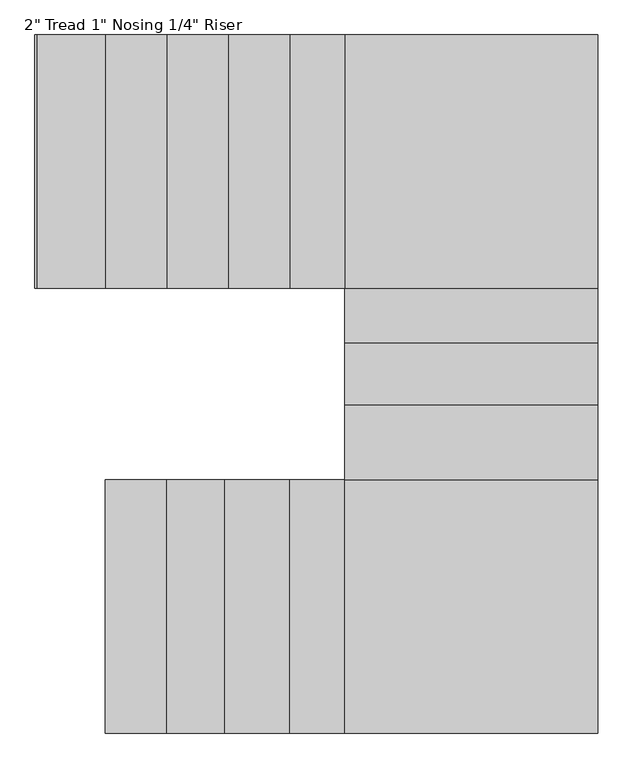
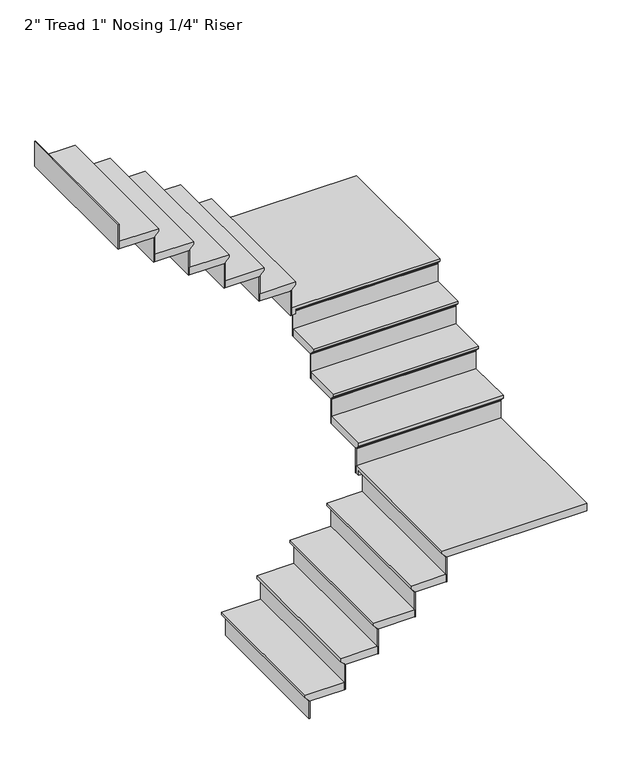
"""IFC4 building model written with IfcOpenShell, lengths in millimetres: stair flight geometry."""

from ifc_helpers import new_model, si_unit, origin, place, context, project, spatial, faceted_brep, source, transform, mapped, element, save


def stair_flight_f19c2654(model_context):
    return source(origin(), model_context, "Body", "Brep", [
        faceted_brep([(344.764115, -6141.1350571, 9751.4833333), (344.764115, -6141.1350571, 9770.5333333), (344.764115, -5201.3350571, 9770.5333333), (344.764115, -5201.3350571, 9751.4833333), (370.164115, -6141.1350571, 9726.0833333), (370.164115, -5201.3350571, 9726.0833333), (598.764115, -6141.1350571, 9770.5333333), (598.764115, -5201.3350571, 9770.5333333), (370.164115, -5201.3350571, 9719.7333333), (598.764115, -5201.3350571, 9719.7333333), (598.764115, -6141.1350571, 9719.7333333), (370.164115, -6141.1350571, 9719.7333333)], [[[0, 1, 2, 3]], [[4, 0, 3, 5]], [[2, 1, 6, 7]], [[8, 9, 10, 11]], [[2, 7, 9, 8, 5, 3]], [[8, 11, 4, 5]], [[6, 1, 0, 4, 11, 10]], [[7, 6, 10, 9]]]),
        faceted_brep([(370.164115, -6141.1350571, 9719.7333333), (370.164115, -6141.1350571, 9601.2), (376.514115, -6141.1350571, 9601.2), (376.514115, -6141.1350571, 9719.7333333), (370.164115, -5201.3350571, 9719.7333333), (376.514115, -5201.3350571, 9719.7333333), (376.514115, -5201.3350571, 9601.2), (370.164115, -5201.3350571, 9601.2)], [[[0, 1, 2, 3]], [[4, 5, 6, 7]], [[1, 0, 4, 7]], [[2, 1, 7, 6]], [[3, 2, 6, 5]], [[0, 3, 5, 4]]]),
        faceted_brep([(598.764115, -6141.1350571, 9889.0666667), (598.764115, -6141.1350571, 9719.7333333), (605.114115, -6141.1350571, 9719.7333333), (605.114115, -6141.1350571, 9889.0666667), (598.764115, -5201.3350571, 9889.0666667), (605.114115, -5201.3350571, 9889.0666667), (605.114115, -5201.3350571, 9719.7333333), (598.764115, -5201.3350571, 9719.7333333)], [[[0, 1, 2, 3]], [[4, 5, 6, 7]], [[1, 0, 4, 7]], [[2, 1, 7, 6]], [[3, 2, 6, 5]], [[0, 3, 5, 4]]]),
        faceted_brep([(573.364115, -5201.3350571, 9939.8666667), (573.364115, -6141.1350571, 9939.8666667), (814.664115, -6141.1350571, 9939.8666667), (814.664115, -5201.3350571, 9939.8666667), (598.764115, -5201.3350571, 9889.0666667), (814.664115, -5201.3350571, 9889.0666667), (814.664115, -6141.1350571, 9889.0666667), (598.764115, -6141.1350571, 9889.0666667), (598.764115, -5201.3350571, 9895.4166667), (573.364115, -5201.3350571, 9920.8166667), (598.764115, -6141.1350571, 9895.4166667), (573.364115, -6141.1350571, 9920.8166667)], [[[0, 1, 2, 3]], [[4, 5, 6, 7]], [[0, 3, 5, 4, 8, 9]], [[4, 7, 10, 8]], [[2, 1, 11, 10, 7, 6]], [[3, 2, 6, 5]], [[11, 1, 0, 9]], [[10, 11, 9, 8]]]),
        faceted_brep([(814.664115, -6141.1350571, 10058.4), (814.664115, -6141.1350571, 9889.0666667), (821.014115, -6141.1350571, 9889.0666667), (821.014115, -6141.1350571, 10058.4), (814.664115, -5201.3350571, 10058.4), (821.014115, -5201.3350571, 10058.4), (821.014115, -5201.3350571, 9889.0666667), (814.664115, -5201.3350571, 9889.0666667)], [[[0, 1, 2, 3]], [[4, 5, 6, 7]], [[1, 0, 4, 7]], [[2, 1, 7, 6]], [[3, 2, 6, 5]], [[0, 3, 5, 4]]]),
        faceted_brep([(789.264115, -5201.3350571, 10109.2), (789.264115, -6141.1350571, 10109.2), (1055.964115, -6141.1350571, 10109.2), (1055.964115, -5201.3350571, 10109.2), (814.664115, -5201.3350571, 10058.4), (1055.964115, -5201.3350571, 10058.4), (1055.964115, -6141.1350571, 10058.4), (814.664115, -6141.1350571, 10058.4), (814.664115, -5201.3350571, 10064.75), (789.264115, -5201.3350571, 10090.15), (814.664115, -6141.1350571, 10064.75), (789.264115, -6141.1350571, 10090.15)], [[[0, 1, 2, 3]], [[4, 5, 6, 7]], [[0, 3, 5, 4, 8, 9]], [[4, 7, 10, 8]], [[2, 1, 11, 10, 7, 6]], [[3, 2, 6, 5]], [[11, 1, 0, 9]], [[10, 11, 9, 8]]]),
        faceted_brep([(1055.964115, -6141.1350571, 10227.7333333), (1055.964115, -6141.1350571, 10058.4), (1062.314115, -6141.1350571, 10058.4), (1062.314115, -6141.1350571, 10227.7333333), (1055.964115, -5201.3350571, 10227.7333333), (1062.314115, -5201.3350571, 10227.7333333), (1062.314115, -5201.3350571, 10058.4), (1055.964115, -5201.3350571, 10058.4)], [[[0, 1, 2, 3]], [[4, 5, 6, 7]], [[1, 0, 4, 7]], [[2, 1, 7, 6]], [[3, 2, 6, 5]], [[0, 3, 5, 4]]]),
        faceted_brep([(1030.564115, -5201.3350571, 10278.5333333), (1030.564115, -6141.1350571, 10278.5333333), (1259.164115, -6141.1350571, 10278.5333333), (1259.164115, -5201.3350571, 10278.5333333), (1055.964115, -5201.3350571, 10227.7333333), (1259.164115, -5201.3350571, 10227.7333333), (1259.164115, -6141.1350571, 10227.7333333), (1055.964115, -6141.1350571, 10227.7333333), (1055.964115, -5201.3350571, 10234.0833333), (1030.564115, -5201.3350571, 10259.4833333), (1055.964115, -6141.1350571, 10234.0833333), (1030.564115, -6141.1350571, 10259.4833333)], [[[0, 1, 2, 3]], [[4, 5, 6, 7]], [[0, 3, 5, 4, 8, 9]], [[4, 7, 10, 8]], [[2, 1, 11, 10, 7, 6]], [[3, 2, 6, 5]], [[11, 1, 0, 9]], [[10, 11, 9, 8]]]),
        faceted_brep([(1259.164115, -6141.1350571, 10397.0666667), (1259.164115, -6141.1350571, 10227.7333333), (1265.514115, -6141.1350571, 10227.7333333), (1265.514115, -6141.1350571, 10397.0666667), (1259.164115, -5201.3350571, 10397.0666667), (1265.514115, -5201.3350571, 10397.0666667), (1265.514115, -5201.3350571, 10227.7333333), (1259.164115, -5201.3350571, 10227.7333333)], [[[0, 1, 2, 3]], [[4, 5, 6, 7]], [[1, 0, 4, 7]], [[2, 1, 7, 6]], [[3, 2, 6, 5]], [[0, 3, 5, 4]]]),
        faceted_brep([(2173.564115, -6141.1350571, 10447.8666667), (2173.564115, -5175.9350571, 10447.8666667), (1233.764115, -5175.9350571, 10447.8666667), (1233.764115, -6141.1350571, 10447.8666667), (1233.764115, -5201.3350571, 10397.0666667), (1233.764115, -5175.9350571, 10397.0666667), (2173.564115, -5175.9350571, 10397.0666667), (2173.564115, -6141.1350571, 10397.0666667), (1259.164115, -6141.1350571, 10397.0666667), (1259.164115, -5201.3350571, 10397.0666667), (1233.764115, -5201.3350571, 10428.8166667), (1233.764115, -6141.1350571, 10428.8166667), (1259.164115, -5201.3350571, 10403.4166667), (1259.164115, -6141.1350571, 10403.4166667)], [[[0, 1, 2, 3]], [[4, 5, 6, 7, 8, 9]], [[3, 2, 5, 4, 10, 11]], [[4, 9, 12, 10]], [[9, 8, 13, 12]], [[0, 3, 11, 13, 8, 7]], [[1, 0, 7, 6]], [[2, 1, 6, 5]], [[13, 11, 10, 12]]]),
        faceted_brep([(2173.564115, -5175.9350571, 10566.4), (2173.564115, -5175.9350571, 10397.0666667), (2173.564115, -5169.5850571, 10397.0666667), (2173.564115, -5169.5850571, 10566.4), (1233.764115, -5175.9350571, 10566.4), (1233.764115, -5169.5850571, 10566.4), (1233.764115, -5169.5850571, 10397.0666667), (1233.764115, -5175.9350571, 10397.0666667)], [[[0, 1, 2, 3]], [[4, 5, 6, 7]], [[1, 0, 4, 7]], [[2, 1, 7, 6]], [[3, 2, 6, 5]], [[0, 3, 5, 4]]]),
        faceted_brep([(1233.764115, -5201.3350571, 10617.2), (2173.564115, -5201.3350571, 10617.2), (2173.564115, -4896.5350571, 10617.2), (1233.764115, -4896.5350571, 10617.2), (1233.764115, -5175.9350571, 10566.4), (1233.764115, -4896.5350571, 10566.4), (2173.564115, -4896.5350571, 10566.4), (2173.564115, -5175.9350571, 10566.4), (1233.764115, -5175.9350571, 10572.75), (1233.764115, -5201.3350571, 10598.15), (2173.564115, -5175.9350571, 10572.75), (2173.564115, -5201.3350571, 10598.15)], [[[0, 1, 2, 3]], [[4, 5, 6, 7]], [[0, 3, 5, 4, 8, 9]], [[4, 7, 10, 8]], [[2, 1, 11, 10, 7, 6]], [[3, 2, 6, 5]], [[11, 1, 0, 9]], [[10, 11, 9, 8]]]),
        faceted_brep([(2173.564115, -4896.5350571, 10735.7333333), (2173.564115, -4896.5350571, 10566.4), (2173.564115, -4890.1850571, 10566.4), (2173.564115, -4890.1850571, 10735.7333333), (1233.764115, -4896.5350571, 10735.7333333), (1233.764115, -4890.1850571, 10735.7333333), (1233.764115, -4890.1850571, 10566.4), (1233.764115, -4896.5350571, 10566.4)], [[[0, 1, 2, 3]], [[4, 5, 6, 7]], [[1, 0, 4, 7]], [[2, 1, 7, 6]], [[3, 2, 6, 5]], [[0, 3, 5, 4]]]),
        faceted_brep([(1233.764115, -4921.9350571, 10786.5333333), (2173.564115, -4921.9350571, 10786.5333333), (2173.564115, -4667.9350571, 10786.5333333), (1233.764115, -4667.9350571, 10786.5333333), (1233.764115, -4896.5350571, 10735.7333333), (1233.764115, -4667.9350571, 10735.7333333), (2173.564115, -4667.9350571, 10735.7333333), (2173.564115, -4896.5350571, 10735.7333333), (1233.764115, -4896.5350571, 10742.0833333), (1233.764115, -4921.9350571, 10767.4833333), (2173.564115, -4896.5350571, 10742.0833333), (2173.564115, -4921.9350571, 10767.4833333)], [[[0, 1, 2, 3]], [[4, 5, 6, 7]], [[0, 3, 5, 4, 8, 9]], [[4, 7, 10, 8]], [[2, 1, 11, 10, 7, 6]], [[3, 2, 6, 5]], [[11, 1, 0, 9]], [[10, 11, 9, 8]]]),
        faceted_brep([(2173.564115, -4667.9350571, 10905.0666667), (2173.564115, -4667.9350571, 10735.7333333), (2173.564115, -4661.5850571, 10735.7333333), (2173.564115, -4661.5850571, 10905.0666667), (1233.764115, -4667.9350571, 10905.0666667), (1233.764115, -4661.5850571, 10905.0666667), (1233.764115, -4661.5850571, 10735.7333333), (1233.764115, -4667.9350571, 10735.7333333)], [[[0, 1, 2, 3]], [[4, 5, 6, 7]], [[1, 0, 4, 7]], [[2, 1, 7, 6]], [[3, 2, 6, 5]], [[0, 3, 5, 4]]]),
        faceted_brep([(1233.764115, -4693.3350571, 10955.8666667), (2173.564115, -4693.3350571, 10955.8666667), (2173.564115, -4464.7350571, 10955.8666667), (1233.764115, -4464.7350571, 10955.8666667), (1233.764115, -4667.9350571, 10905.0666667), (1233.764115, -4464.7350571, 10905.0666667), (2173.564115, -4464.7350571, 10905.0666667), (2173.564115, -4667.9350571, 10905.0666667), (1233.764115, -4667.9350571, 10911.4166667), (1233.764115, -4693.3350571, 10936.8166667), (2173.564115, -4667.9350571, 10911.4166667), (2173.564115, -4693.3350571, 10936.8166667)], [[[0, 1, 2, 3]], [[4, 5, 6, 7]], [[0, 3, 5, 4, 8, 9]], [[4, 7, 10, 8]], [[2, 1, 11, 10, 7, 6]], [[3, 2, 6, 5]], [[11, 1, 0, 9]], [[10, 11, 9, 8]]]),
        faceted_brep([(2173.564115, -4464.7350571, 11074.4), (2173.564115, -4464.7350571, 10905.0666667), (2173.564115, -4458.3850571, 10905.0666667), (2173.564115, -4458.3850571, 11074.4), (1233.764115, -4464.7350571, 11074.4), (1233.764115, -4458.3850571, 11074.4), (1233.764115, -4458.3850571, 10905.0666667), (1233.764115, -4464.7350571, 10905.0666667)], [[[0, 1, 2, 3]], [[4, 5, 6, 7]], [[1, 0, 4, 7]], [[2, 1, 7, 6]], [[3, 2, 6, 5]], [[0, 3, 5, 4]]]),
        faceted_brep([(2173.564115, -3550.3350571, 11125.2), (1208.364115, -3550.3350571, 11125.2), (1208.364115, -4490.1350571, 11125.2), (2173.564115, -4490.1350571, 11125.2), (1233.764115, -4490.1350571, 11074.4), (1208.364115, -4490.1350571, 11074.4), (1208.364115, -3550.3350571, 11074.4), (2173.564115, -3550.3350571, 11074.4), (2173.564115, -4464.7350571, 11074.4), (1233.764115, -4464.7350571, 11074.4), (1233.764115, -4490.1350571, 11106.15), (2173.564115, -4490.1350571, 11106.15), (1233.764115, -4464.7350571, 11080.75), (2173.564115, -4464.7350571, 11080.75)], [[[0, 1, 2, 3]], [[4, 5, 6, 7, 8, 9]], [[3, 2, 5, 4, 10, 11]], [[4, 9, 12, 10]], [[9, 8, 13, 12]], [[0, 3, 11, 13, 8, 7]], [[1, 0, 7, 6]], [[2, 1, 6, 5]], [[13, 11, 10, 12]]]),
        faceted_brep([(1208.364115, -3550.3350571, 11243.7333333), (1208.364115, -3550.3350571, 11074.4), (1202.014115, -3550.3350571, 11074.4), (1202.014115, -3550.3350571, 11243.7333333), (1208.364115, -4490.1350571, 11243.7333333), (1202.014115, -4490.1350571, 11243.7333333), (1202.014115, -4490.1350571, 11074.4), (1208.364115, -4490.1350571, 11074.4)], [[[0, 1, 2, 3]], [[4, 5, 6, 7]], [[1, 0, 4, 7]], [[2, 1, 7, 6]], [[3, 2, 6, 5]], [[0, 3, 5, 4]]]),
        faceted_brep([(1233.764115, -4490.1350571, 11294.5333333), (1233.764115, -3550.3350571, 11294.5333333), (1005.164115, -3550.3350571, 11294.5333333), (1005.164115, -4490.1350571, 11294.5333333), (1208.364115, -4490.1350571, 11243.7333333), (1005.164115, -4490.1350571, 11243.7333333), (1005.164115, -3550.3350571, 11243.7333333), (1208.364115, -3550.3350571, 11243.7333333), (1208.364115, -4490.1350571, 11250.0833333), (1233.764115, -4490.1350571, 11275.4833333), (1208.364115, -3550.3350571, 11250.0833333), (1233.764115, -3550.3350571, 11275.4833333)], [[[0, 1, 2, 3]], [[4, 5, 6, 7]], [[0, 3, 5, 4, 8, 9]], [[4, 7, 10, 8]], [[2, 1, 11, 10, 7, 6]], [[3, 2, 6, 5]], [[11, 1, 0, 9]], [[10, 11, 9, 8]]]),
        faceted_brep([(1005.164115, -3550.3350571, 11413.0666667), (1005.164115, -3550.3350571, 11243.7333333), (998.814115, -3550.3350571, 11243.7333333), (998.814115, -3550.3350571, 11413.0666667), (1005.164115, -4490.1350571, 11413.0666667), (998.814115, -4490.1350571, 11413.0666667), (998.814115, -4490.1350571, 11243.7333333), (1005.164115, -4490.1350571, 11243.7333333)], [[[0, 1, 2, 3]], [[4, 5, 6, 7]], [[1, 0, 4, 7]], [[2, 1, 7, 6]], [[3, 2, 6, 5]], [[0, 3, 5, 4]]]),
        faceted_brep([(1030.564115, -4490.1350571, 11463.8666667), (1030.564115, -3550.3350571, 11463.8666667), (776.564115, -3550.3350571, 11463.8666667), (776.564115, -4490.1350571, 11463.8666667), (1005.164115, -4490.1350571, 11413.0666667), (776.564115, -4490.1350571, 11413.0666667), (776.564115, -3550.3350571, 11413.0666667), (1005.164115, -3550.3350571, 11413.0666667), (1005.164115, -4490.1350571, 11419.4166667), (1030.564115, -4490.1350571, 11444.8166667), (1005.164115, -3550.3350571, 11419.4166667), (1030.564115, -3550.3350571, 11444.8166667)], [[[0, 1, 2, 3]], [[4, 5, 6, 7]], [[0, 3, 5, 4, 8, 9]], [[4, 7, 10, 8]], [[2, 1, 11, 10, 7, 6]], [[3, 2, 6, 5]], [[11, 1, 0, 9]], [[10, 11, 9, 8]]]),
        faceted_brep([(776.564115, -3550.3350571, 11582.4), (776.564115, -3550.3350571, 11413.0666667), (770.214115, -3550.3350571, 11413.0666667), (770.214115, -3550.3350571, 11582.4), (776.564115, -4490.1350571, 11582.4), (770.214115, -4490.1350571, 11582.4), (770.214115, -4490.1350571, 11413.0666667), (776.564115, -4490.1350571, 11413.0666667)], [[[0, 1, 2, 3]], [[4, 5, 6, 7]], [[1, 0, 4, 7]], [[2, 1, 7, 6]], [[3, 2, 6, 5]], [[0, 3, 5, 4]]]),
        faceted_brep([(801.964115, -4490.1350571, 11633.2), (801.964115, -3550.3350571, 11633.2), (547.964115, -3550.3350571, 11633.2), (547.964115, -4490.1350571, 11633.2), (776.564115, -4490.1350571, 11582.4), (547.964115, -4490.1350571, 11582.4), (547.964115, -3550.3350571, 11582.4), (776.564115, -3550.3350571, 11582.4), (776.564115, -4490.1350571, 11588.75), (801.964115, -4490.1350571, 11614.15), (776.564115, -3550.3350571, 11588.75), (801.964115, -3550.3350571, 11614.15)], [[[0, 1, 2, 3]], [[4, 5, 6, 7]], [[0, 3, 5, 4, 8, 9]], [[4, 7, 10, 8]], [[2, 1, 11, 10, 7, 6]], [[3, 2, 6, 5]], [[11, 1, 0, 9]], [[10, 11, 9, 8]]]),
        faceted_brep([(547.964115, -3550.3350571, 11751.7333333), (547.964115, -3550.3350571, 11582.4), (541.614115, -3550.3350571, 11582.4), (541.614115, -3550.3350571, 11751.7333333), (547.964115, -4490.1350571, 11751.7333333), (541.614115, -4490.1350571, 11751.7333333), (541.614115, -4490.1350571, 11582.4), (547.964115, -4490.1350571, 11582.4)], [[[0, 1, 2, 3]], [[4, 5, 6, 7]], [[1, 0, 4, 7]], [[2, 1, 7, 6]], [[3, 2, 6, 5]], [[0, 3, 5, 4]]]),
        faceted_brep([(573.364115, -4490.1350571, 11802.5333333), (573.364115, -3550.3350571, 11802.5333333), (319.364115, -3550.3350571, 11802.5333333), (319.364115, -4490.1350571, 11802.5333333), (547.964115, -4490.1350571, 11751.7333333), (319.364115, -4490.1350571, 11751.7333333), (319.364115, -3550.3350571, 11751.7333333), (547.964115, -3550.3350571, 11751.7333333), (547.964115, -4490.1350571, 11758.0833333), (573.364115, -4490.1350571, 11783.4833333), (547.964115, -3550.3350571, 11758.0833333), (573.364115, -3550.3350571, 11783.4833333)], [[[0, 1, 2, 3]], [[4, 5, 6, 7]], [[0, 3, 5, 4, 8, 9]], [[4, 7, 10, 8]], [[2, 1, 11, 10, 7, 6]], [[3, 2, 6, 5]], [[11, 1, 0, 9]], [[10, 11, 9, 8]]]),
        faceted_brep([(319.364115, -3550.3350571, 11921.0666667), (319.364115, -3550.3350571, 11751.7333333), (313.014115, -3550.3350571, 11751.7333333), (313.014115, -3550.3350571, 11921.0666667), (319.364115, -4490.1350571, 11921.0666667), (313.014115, -4490.1350571, 11921.0666667), (313.014115, -4490.1350571, 11751.7333333), (319.364115, -4490.1350571, 11751.7333333)], [[[0, 1, 2, 3]], [[4, 5, 6, 7]], [[1, 0, 4, 7]], [[2, 1, 7, 6]], [[3, 2, 6, 5]], [[0, 3, 5, 4]]]),
        faceted_brep([(90.764115, -3550.3350571, 12090.4), (90.764115, -3550.3350571, 11921.0666667), (84.414115, -3550.3350571, 11921.0666667), (84.414115, -3550.3350571, 12090.4), (90.764115, -4490.1350571, 12090.4), (84.414115, -4490.1350571, 12090.4), (84.414115, -4490.1350571, 11921.0666667), (90.764115, -4490.1350571, 11921.0666667)], [[[0, 1, 2, 3]], [[4, 5, 6, 7]], [[1, 0, 4, 7]], [[2, 1, 7, 6]], [[3, 2, 6, 5]], [[0, 3, 5, 4]]]),
        faceted_brep([(344.764115, -4490.1350571, 11971.8666667), (344.764115, -3550.3350571, 11971.8666667), (90.764115, -3550.3350571, 11971.8666667), (90.764115, -4490.1350571, 11971.8666667), (319.364115, -4490.1350571, 11921.0666667), (90.764115, -4490.1350571, 11921.0666667), (90.764115, -3550.3350571, 11921.0666667), (319.364115, -3550.3350571, 11921.0666667), (319.364115, -4490.1350571, 11927.4166667), (344.764115, -4490.1350571, 11952.8166667), (319.364115, -3550.3350571, 11927.4166667), (344.764115, -3550.3350571, 11952.8166667)], [[[0, 1, 2, 3]], [[4, 5, 6, 7]], [[0, 3, 5, 4, 8, 9]], [[4, 7, 10, 8]], [[2, 1, 11, 10, 7, 6]], [[3, 2, 6, 5]], [[11, 1, 0, 9]], [[10, 11, 9, 8]]]),
    ])


if __name__ == "__main__":
    model = new_model("IFC4")
    model_context = context("Model", 3, world=origin())
    ifc_project = project(units=[si_unit("LENGTHUNIT", "METRE", prefix="MILLI")], contexts=[model_context])
    site = spatial("IfcSite", under=ifc_project)
    building = spatial("IfcBuilding", under=site)
    placement = place(None, origin())
    stair_flight_shape = stair_flight_f19c2654(model_context)
    element("IfcStairFlight", 1, ObjectType="2\" Tread 1\" Nosing 1/4\" Riser", at=placement, inside=building, context=model_context, shape_type="MappedRepresentation", body=[
        mapped(stair_flight_shape, transform((0.0, 0.0, 0.0), x_axis=(1.0, 0.0, 0.0), y_axis=(0.0, 1.0, 0.0), z_axis=(0.0, 0.0, 1.0))),
    ])
    save(model, "model.ifc")
